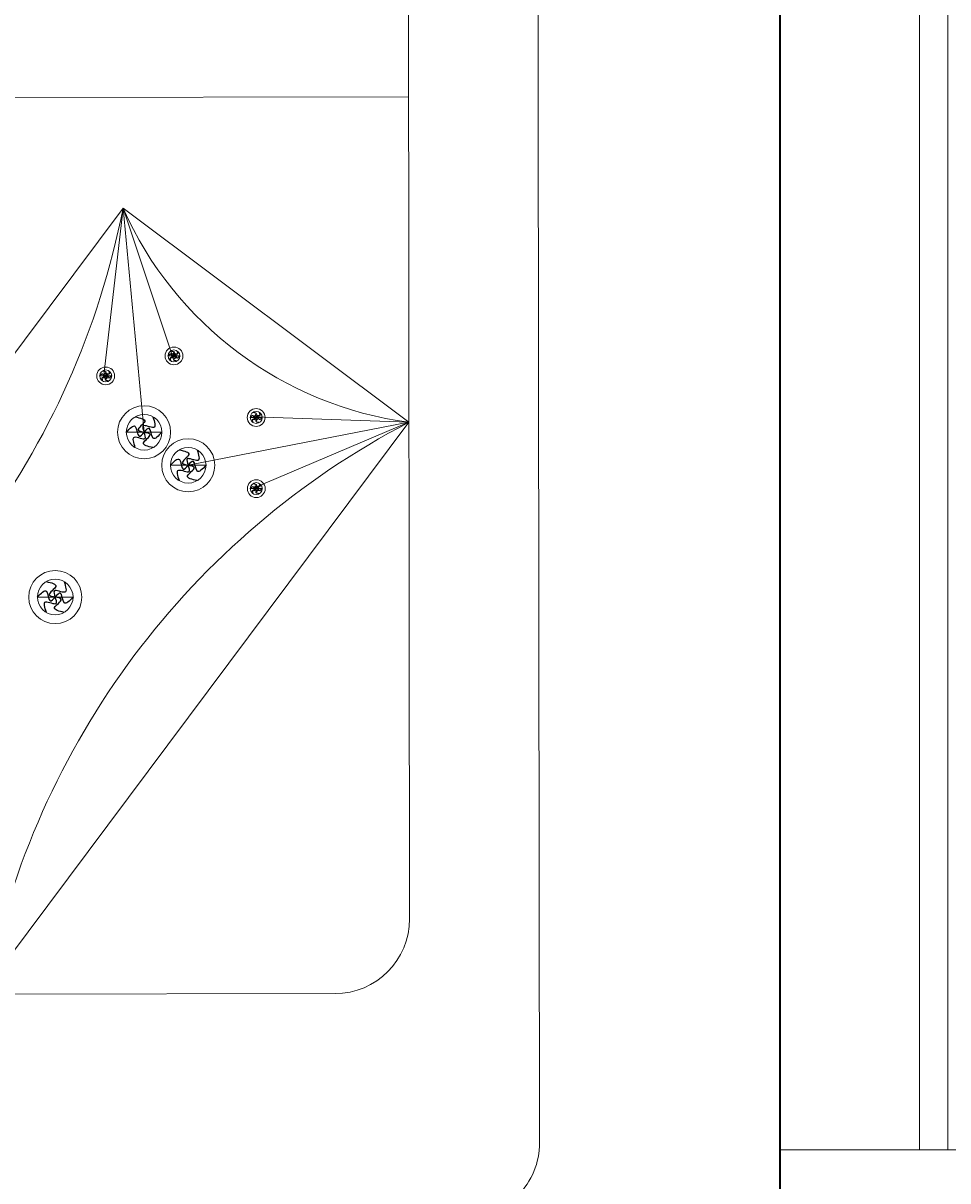
# Model space of a CAD drawing. Units: inches. Extents: x -61 to 1599, y -1316 to 257.
# Tile 137 of 204: x 515 to 540, y -135 to -104. Entities that reach past the tile are written whole.
import ezdxf

# ---------------------------------------------------------------- set-up
doc = ezdxf.new("R2010")
doc.units = ezdxf.units.IN
doc.header["$MEASUREMENT"] = 0
for name, color, linetype, lineweight in [('A-ANNO-DIMS', 2, 'Continuous', 18), ('FURNITURE', 83, 'Continuous', 18), ('WALLS', 4, 'Continuous', 35), ('WINDOWS', 220, 'Continuous', 18)]:
    doc.layers.add(name, color=color, linetype=linetype, lineweight=lineweight)
doc.layers.add('FUR', color=83, linetype='Continuous')
doc.styles.get("Standard").update_dxf_attribs({"font": 'arial.ttf'})
doc.dimstyles.get("Standard").update_dxf_attribs({"dimtxt": 0.18, "dimasz": 0.18, "dimexe": 0.18, "dimexo": 0.0625, "dimgap": 0.09, "dimtad": 0, "dimtih": 1, "dimtoh": 1, "dimdec": 0, "dimzin": 0, "dimdsep": 46, "dimlunit": 3, "dimtxsty": 'Standard', "dimcen": 0.09, "dimadec": 0, "dimazin": 0, "dimtfac": 1, "dimtdec": 0, "dimtofl": 0, "dimtmove": 0, "dimatfit": 3, "dimfxl": 1, "dimtolj": 1, "dimtzin": 0, "dimarcsym": 0})

# ---------------------------------------------------------------- blocks, each defined once
blk = doc.blocks.new('*U219')
at = {"layer": 'FUR'}
blk.add_open_spline([(0.015, 0.238), (-0.088, 0.143), (-0.292, -0.045), (0.224, -0.053), (0.072, -0.187), (0.015, -0.238)], degree=3, knots=[0, 0, 0, 0, 0.2846533, 0.5662105, 0.736751, 0.736751, 0.736751, 0.736751], dxfattribs=at)
blk = doc.blocks.new('*U220')
at = {"layer": 'FURNITURE', "transparency": 16777216}
for p, rotation in [((662.517, -238.489), 60), ((662.929, -238.463), 300), ((662.531, -238.727), 120), ((662.944, -238.702), 240), ((662.745, -238.833), 180)]:
    blk.add_blockref('*U219', p, dxfattribs=dict(at, rotation=rotation))
blk.add_blockref('*U219', (662.716, -238.357), dxfattribs=at)
blk = doc.blocks.new('*U233')
at = {"layer": 'FUR'}
blk.add_open_spline([(0.015, 0.238), (-0.088, 0.143), (-0.292, -0.045), (0.224, -0.053), (0.072, -0.187), (0.015, -0.238)], degree=3, knots=[0, 0, 0, 0, 0.2846533, 0.5662105, 0.736751, 0.736751, 0.736751, 0.736751], dxfattribs=at)
blk = doc.blocks.new('*U253')
at = {"layer": 'FURNITURE', "transparency": 16777216}
for p, rotation in [((662.517, -238.489), 60), ((662.929, -238.463), 300), ((662.531, -238.727), 120), ((662.944, -238.702), 240), ((662.745, -238.833), 180)]:
    blk.add_blockref('*U233', p, dxfattribs=dict(at, rotation=rotation))
blk.add_blockref('*U233', (662.716, -238.357), dxfattribs=at)
blk = doc.blocks.new('*U254')
at = {"layer": 'FUR'}
blk.add_open_spline([(0.005, 0.08), (-0.03, 0.048), (-0.098, -0.015), (0.075, -0.018), (0.024, -0.063), (0.005, -0.08)], degree=3, knots=[0, 0, 0, 0, 0.0954578, 0.1898773, 0.2470677, 0.2470677, 0.2470677, 0.2470677], dxfattribs=at)
blk = doc.blocks.new('*U255')
at = {"layer": 'FURNITURE', "transparency": 16777216}
for p, rotation in [((222.173, -79.977), 60), ((222.312, -79.968), 300), ((222.178, -80.056), 120), ((222.25, -80.092), 180), ((222.317, -80.048), 240)]:
    blk.add_blockref('*U254', p, dxfattribs=dict(at, rotation=rotation))
blk.add_blockref('*U254', (222.24, -79.932), dxfattribs=at)
blk = doc.blocks.new('*U221')
at = {"layer": 'FUR'}
blk.add_open_spline([(0.005, 0.08), (-0.03, 0.048), (-0.098, -0.015), (0.075, -0.018), (0.024, -0.063), (0.005, -0.08)], degree=3, knots=[0, 0, 0, 0, 0.0954578, 0.1898773, 0.2470677, 0.2470677, 0.2470677, 0.2470677], dxfattribs=at)
blk = doc.blocks.new('*U222')
at = {"layer": 'FURNITURE', "transparency": 16777216}
for p, rotation in [((222.173, -79.977), 60), ((222.312, -79.968), 300), ((222.178, -80.056), 120), ((222.25, -80.092), 180), ((222.317, -80.048), 240)]:
    blk.add_blockref('*U221', p, dxfattribs=dict(at, rotation=rotation))
blk.add_blockref('*U221', (222.24, -79.932), dxfattribs=at)
blk = doc.blocks.new('*U223')
at = {"layer": 'FUR'}
blk.add_open_spline([(0.005, 0.08), (-0.03, 0.048), (-0.098, -0.015), (0.075, -0.018), (0.024, -0.063), (0.005, -0.08)], degree=3, knots=[0, 0, 0, 0, 0.0954578, 0.1898773, 0.2470677, 0.2470677, 0.2470677, 0.2470677], dxfattribs=at)
blk = doc.blocks.new('*U224')
at = {"layer": 'FURNITURE', "transparency": 16777216}
for p, rotation in [((222.173, -79.977), 60), ((222.312, -79.968), 300), ((222.178, -80.056), 120), ((222.25, -80.092), 180), ((222.317, -80.048), 240)]:
    blk.add_blockref('*U223', p, dxfattribs=dict(at, rotation=rotation))
blk.add_blockref('*U223', (222.24, -79.932), dxfattribs=at)
blk = doc.blocks.new('*U225')
at = {"layer": 'FUR'}
blk.add_open_spline([(0.005, 0.08), (-0.03, 0.048), (-0.098, -0.015), (0.075, -0.018), (0.024, -0.063), (0.005, -0.08)], degree=3, knots=[0, 0, 0, 0, 0.0954578, 0.1898773, 0.2470677, 0.2470677, 0.2470677, 0.2470677], dxfattribs=at)
blk = doc.blocks.new('*U226')
at = {"layer": 'FURNITURE', "transparency": 16777216}
for p, rotation in [((222.173, -79.977), 60), ((222.312, -79.968), 300), ((222.178, -80.056), 120), ((222.25, -80.092), 180), ((222.317, -80.048), 240)]:
    blk.add_blockref('*U225', p, dxfattribs=dict(at, rotation=rotation))
blk.add_blockref('*U225', (222.24, -79.932), dxfattribs=at)
blk = doc.blocks.new('*U262')
at = {"layer": 'FUR'}
blk.add_open_spline([(0.015, 0.238), (-0.088, 0.143), (-0.292, -0.045), (0.224, -0.053), (0.072, -0.187), (0.015, -0.238)], degree=3, knots=[0, 0, 0, 0, 0.2846533, 0.5662105, 0.736751, 0.736751, 0.736751, 0.736751], dxfattribs=at)
blk = doc.blocks.new('*U218')
at = {"layer": 'FURNITURE', "transparency": 16777216}
for p, rotation in [((662.517, -238.489), 60), ((662.929, -238.463), 300), ((662.531, -238.727), 120), ((662.944, -238.702), 240), ((662.745, -238.833), 180)]:
    blk.add_blockref('*U262', p, dxfattribs=dict(at, rotation=rotation))
blk.add_blockref('*U262', (662.716, -238.357), dxfattribs=at)
blk = doc.blocks.new('WIN-36IN')
for p, q in [((0, 4.5), (0, 9)), ((0, 9), (0, 0)), ((0, 5.262), (36, 5.262)), ((0, 4.5), (36, 4.5)), ((0, 4.5), (36, 4.5))]:
    blk.add_line(p, q)
blk = doc.blocks.new('*D704')
at = {"layer": 'A-ANNO-DIMS', "color": 0, "lineweight": -2, "transparency": 16777216}
for p, q in [((491.833, -616.882), (491.833, 257.457)), ((492.013, 257.277), (517.874, 257.277)), ((544.523, 257.277), (518.661, 257.277)), ((544.703, -616.882), (544.703, 257.457))]:
    blk.add_line(p, q, dxfattribs=at)
at = {"layer": 'A-ANNO-DIMS', "color": 0, "transparency": 16777216}
for points in [[(492.013, 257.307), (492.013, 257.247), (491.833, 257.277)], [(544.523, 257.307), (544.523, 257.247), (544.703, 257.277)]]:
    blk.add_solid(points, dxfattribs=at)
at = {"layer": 'DEFPOINTS', "color": 0, "transparency": 16777216}
for p in [(544.703, 257.277), (491.833, -616.945), (544.703, -616.945)]:
    blk.add_point(p, dxfattribs=at)
at = {"layer": 'A-ANNO-DIMS', "color": 0, "transparency": 16777216, "insert": (518.268, 257.277), "char_height": 0.18, "attachment_point": 5}
blk.add_mtext('\\A1;52.87', dxfattribs=at)

msp = doc.modelspace()

# ---------------------------------------------------------------- linework, layer by layer
at = {"layer": 'FURNITURE'}
for p, q in [((525.7931, -127.7888), (525.7326, -83.7888)), ((506.7909, -105.8149), (525.7629, -105.7888)), ((518.121, -108.7733), (517.6042, -113.2397)), ((518.121, -108.7733), (518.6848, -114.7666)), ((518.121, -108.7733), (519.4317, -112.7051)), ((519.4842, -112.7244), (519.3244, -112.7246)), ((519.4842, -112.7244), (519.644, -112.7242)), ((517.6567, -113.259), (517.4969, -113.2592)), ((517.6567, -113.259), (517.8165, -113.2588)), ((525.7748, -114.5007), (519.8659, -115.6503)), ((521.6854, -114.3716), (521.5256, -114.3718)), ((525.7748, -114.5007), (521.6329, -114.3523)), ((525.7748, -114.5007), (521.6355, -116.2564)), ((521.6854, -114.3716), (521.8452, -114.3713)), ((518.6848, -114.7666), (518.2084, -114.7672)), ((518.6848, -114.7666), (519.1613, -114.7659)), ((519.8659, -115.6503), (519.3894, -115.651)), ((519.8659, -115.6503), (520.3424, -115.6497)), ((521.688, -116.2757), (521.5283, -116.2759)), ((521.688, -116.2757), (521.8478, -116.2755)), ((516.3055, -119.1773), (515.829, -119.1779)), ((516.3055, -119.1773), (516.782, -119.1766)), ((506.8239, -129.8148), (523.7958, -129.7915))]:
    msp.add_line(p, q, dxfattribs=at)
msp.add_lwpolyline([(503.2659, -129.8197), (503.2714, -133.8197, 0.4142136), (505.2742, -135.817), (527.2741, -135.7867, 0.4142137), (529.2714, -133.784), (529.1944, -77.784, 0.4142134), (527.1916, -75.7868), (505.1917, -75.817, 0.4142136), (503.1944, -77.8197), (503.1999, -81.8197)], format="xyb", dxfattribs=at)
msp.add_lwpolyline([(518.121, -108.7733), (506.8361, -123.8538), (514.49, -129.5812), (525.7748, -114.5007)], close=True, dxfattribs=at)
for centre, radius in [((519.4842, -112.7244), 0.2382), ((519.4842, -112.7244), 0.1598), ((517.6567, -113.259), 0.2382), ((517.6567, -113.259), 0.1598), ((518.6848, -114.7666), 0.7104), ((518.6848, -114.7666), 0.4765), ((521.6854, -114.3716), 0.2382), ((521.6854, -114.3716), 0.1598), ((519.8659, -115.6503), 0.7104), ((519.8659, -115.6503), 0.4765), ((521.688, -116.2757), 0.2382), ((521.688, -116.2757), 0.1598), ((516.3055, -119.1773), 0.7104), ((516.3055, -119.1773), 0.4765)]:
    msp.add_circle(centre, radius, dxfattribs=at)
for centre, radius, start, end in [((496.7984, -104.58), 21.731, 297.51039, 348.87432), ((527.0847, -104.7725), 9.816, 204.05298, 262.33173), ((535.8126, -133.7745), 21.731, 117.51039, 168.87432), ((523.7931, -127.7915), 2, 270.07876, 0.07875)]:
    msp.add_arc(centre, radius, start, end, dxfattribs=at)
at = {"layer": 'WALLS'}
msp.add_line((535.7028, -13.3229), (535.7028, -175.3229), dxfattribs=at)

# ---------------------------------------------------------------- block references
at = {"layer": 'FURNITURE', "xscale": -1, "rotation": 270.0787636990076}
for name, p in [('*U224', (599.802, -334.8591)), ('*U226', (597.9744, -335.3938)), ('*U218', (758.1909, -777.1681)), ('*U222', (602.0032, -336.5063)), ('*U253', (759.3719, -778.0518)), ('*U255', (602.0058, -338.4105)), ('*U220', (755.8115, -781.5788))]:
    msp.add_blockref(name, p, dxfattribs=at)
at = {"layer": 'WINDOWS', "rotation": 90.00000000000011}
msp.add_blockref('WIN-36IN', (544.7029, -133.972), dxfattribs=at)

# ---------------------------------------------------------------- dimensions: what is measured, and where the dimension line sits
at = {"layer": 'A-ANNO-DIMS'}
dim = msp.add_linear_dim(base=(544.7028, 257.2771), p1=(491.8327, -616.9446), p2=(544.7028, -616.9446), dimstyle='Standard', override={"dimdec": 2, "dimlfac": 1, "dimrnd": 0, "dimzin": 0, "dimdsep": 46, "dimlunit": 2}, dxfattribs=at)
dim.commit()
dim.dimension.update_dxf_attribs({"geometry": '*D704', "text_midpoint": (518.2677, 257.2771)})

doc.saveas('drawing.dxf')
